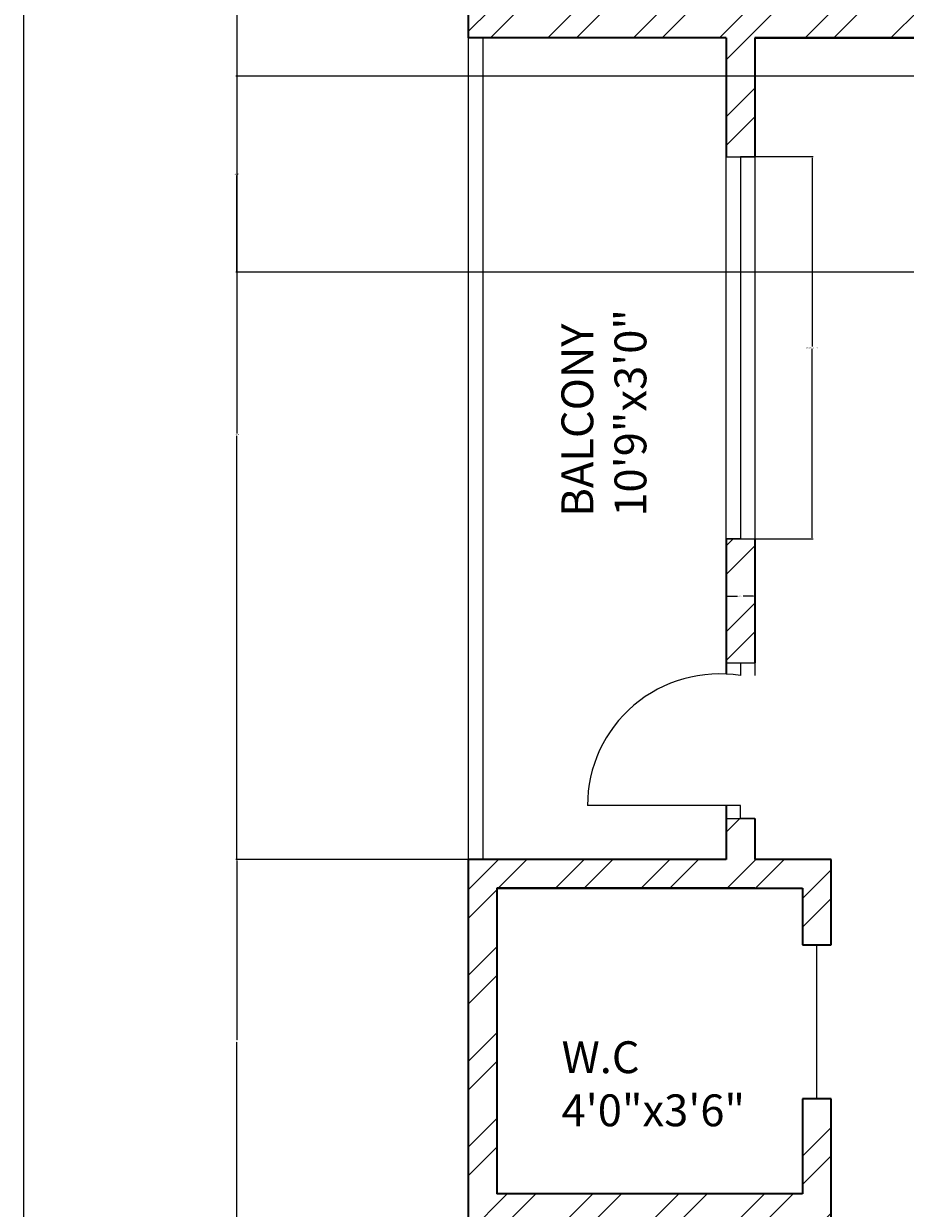
# Model space of a CAD drawing. Units: inches. Extents: x 1570 to 2186, y 1575 to 2421.
# Tile 2 of 10: x 1570 to 1708, y 1859 to 2045. Entities that reach past the tile are written whole.
import ezdxf

# ---------------------------------------------------------------- set-up
doc = ezdxf.new("R2010")
doc.units = ezdxf.units.IN
for name, color, linetype, lineweight in [('A-ANNO-DIMS', 2, 'Continuous', 18), ('A-ANNO-TTLB', 7, 'Continuous', 25), ('A-AREA-IDEN', 7, 'Continuous', 18), ('A-DOOR', 201, 'Continuous', 18), ('A-FLOR-HRAL', 201, 'Continuous', 18), ('A-GLAZ', 150, 'Continuous', 18), ('A-WALL', 7, 'Continuous', 35), ('A-WALL-PATT', 252, 'Continuous', 13)]:
    doc.layers.add(name, color=color, linetype=linetype, lineweight=lineweight)
doc.styles.get("Standard").update_dxf_attribs({"font": 'arial.ttf'})
doc.dimstyles.get("Standard").update_dxf_attribs({"dimtxt": 0.18, "dimasz": 0.18, "dimexe": 0.18, "dimexo": 0.0625, "dimgap": 0.09, "dimtad": 0, "dimtih": 1, "dimtoh": 1, "dimdec": 4, "dimzin": 0, "dimdsep": 46, "dimtxsty": 'Standard', "dimcen": 0.09, "dimadec": 0, "dimazin": 0, "dimtfac": 1, "dimtdec": 4, "dimtofl": 0, "dimtmove": 0, "dimatfit": 3, "dimfxl": 1, "dimtolj": 1, "dimtzin": 0, "dimarcsym": 0})

# ---------------------------------------------------------------- blocks, each defined once
blk = doc.blocks.new('WIN-60IN')
for p, q in [((0, 60), (4.5, 60)), ((0, 0), (0, 60)), ((4.5, 60), (2.25, 60)), ((2.25, 60), (2.25, 0)), ((4.5, 60), (4.5, 0)), ((2.25, 0), (0, 0)), ((0, 0), (4.5, 0))]:
    blk.add_line(p, q)
blk = doc.blocks.new('*D10')
at = {"layer": 'A-ANNO-DIMS', "color": 0, "lineweight": -2, "transparency": 16777216}
for p, q in [((1684.65, 2024.08), (1693.77, 2024.08)), ((1693.59, 2023.9), (1693.59, 1994.26)), ((1693.59, 1964.26), (1693.59, 1993.89)), ((1684.65, 1964.08), (1693.77, 1964.08))]:
    blk.add_line(p, q, dxfattribs=at)
at = {"layer": 'A-ANNO-DIMS', "color": 0, "transparency": 16777216}
for points in [[(1693.56, 2023.9), (1693.62, 2023.9), (1693.59, 2024.08)], [(1693.56, 1964.26), (1693.62, 1964.26), (1693.59, 1964.08)]]:
    blk.add_solid(points, dxfattribs=at)
at = {"layer": 'Defpoints', "color": 0, "transparency": 16777216}
for p in [(1684.59, 2024.08), (1693.59, 2024.08), (1684.59, 1964.08)]:
    blk.add_point(p, dxfattribs=at)
at = {"layer": 'A-ANNO-DIMS', "color": 0, "transparency": 16777216, "insert": (1693.59, 1994.08), "char_height": 0.18, "attachment_point": 5}
blk.add_mtext('\\A1;WINDOW 60 TYP.', dxfattribs=at)
blk = doc.blocks.new('*D11')
at = {"layer": 'A-ANNO-DIMS', "color": 0, "lineweight": -2, "transparency": 16777216}
for p, q in [((1680.09, 1964.01), (1680.09, 1954.9)), ((1684.59, 1964.01), (1684.59, 1954.9)), ((1680.27, 1955.08), (1681.88, 1955.08)), ((1684.41, 1955.08), (1682.8, 1955.08))]:
    blk.add_line(p, q, dxfattribs=at)
at = {"layer": 'A-ANNO-DIMS', "color": 0, "transparency": 16777216}
for points in [[(1680.27, 1955.11), (1680.27, 1955.05), (1680.09, 1955.08)], [(1684.41, 1955.11), (1684.41, 1955.05), (1684.59, 1955.08)]]:
    blk.add_solid(points, dxfattribs=at)
at = {"layer": 'Defpoints', "color": 0, "transparency": 16777216}
for p in [(1680.09, 1964.08), (1684.59, 1964.08), (1684.59, 1955.08)]:
    blk.add_point(p, dxfattribs=at)
at = {"layer": 'A-ANNO-DIMS', "color": 0, "transparency": 16777216, "insert": (1682.34, 1955.08), "char_height": 0.18, "attachment_point": 5}
blk.add_mtext('\\A1;5 TYP.', dxfattribs=at)
blk = doc.blocks.new('*D34')
at = {"layer": 'A-ANNO-DIMS', "color": 0, "lineweight": -2, "transparency": 16777216}
for p, q in [((1639.53, 1913.75), (1603.11, 1913.75)), ((1603.29, 1913.57), (1603.29, 1885.43)), ((1603.29, 1856.93), (1603.29, 1885.07)), ((1639.53, 1856.75), (1603.11, 1856.75))]:
    blk.add_line(p, q, dxfattribs=at)
at = {"layer": 'A-ANNO-DIMS', "color": 0, "transparency": 16777216}
for points in [[(1603.26, 1913.57), (1603.32, 1913.57), (1603.29, 1913.75)], [(1603.26, 1856.93), (1603.32, 1856.93), (1603.29, 1856.75)]]:
    blk.add_solid(points, dxfattribs=at)
at = {"layer": 'Defpoints', "color": 0, "transparency": 16777216}
for p in [(1603.29, 1913.75), (1639.59, 1913.75), (1639.59, 1856.75)]:
    blk.add_point(p, dxfattribs=at)
at = {"layer": 'A-ANNO-DIMS', "color": 0, "transparency": 16777216, "insert": (1603.29, 1885.25), "char_height": 0.18, "attachment_point": 5}
blk.add_mtext('\\A1;57', dxfattribs=at)
blk = doc.blocks.new('*D35')
at = {"layer": 'A-ANNO-DIMS', "color": 0, "lineweight": -2, "transparency": 16777216}
for p, q in [((1639.53, 2047.15), (1603.11, 2047.15)), ((1603.29, 2046.97), (1603.29, 1980.63)), ((1603.29, 1913.93), (1603.29, 1980.27)), ((1639.53, 1913.75), (1603.11, 1913.75))]:
    blk.add_line(p, q, dxfattribs=at)
at = {"layer": 'A-ANNO-DIMS', "color": 0, "transparency": 16777216}
for points in [[(1603.26, 2046.97), (1603.32, 2046.97), (1603.29, 2047.15)], [(1603.26, 1913.93), (1603.32, 1913.93), (1603.29, 1913.75)]]:
    blk.add_solid(points, dxfattribs=at)
at = {"layer": 'Defpoints', "color": 0, "transparency": 16777216}
for p in [(1603.29, 2047.15), (1639.59, 2047.15), (1639.59, 1913.75)]:
    blk.add_point(p, dxfattribs=at)
at = {"layer": 'A-ANNO-DIMS', "color": 0, "transparency": 16777216, "insert": (1603.29, 1980.45), "char_height": 0.18, "attachment_point": 5}
blk.add_mtext('\\A1;133.4', dxfattribs=at)
blk = doc.blocks.new('*D43')
at = {"layer": 'A-ANNO-DIMS', "color": 0, "lineweight": -2, "transparency": 16777216}
for p, q in [((1913.53, 2036.69), (1603.11, 2036.69)), ((1603.29, 2036.51), (1603.29, 2021.49)), ((1603.29, 2006.11), (1603.29, 2021.13)), ((1913.53, 2005.93), (1603.11, 2005.93))]:
    blk.add_line(p, q, dxfattribs=at)
at = {"layer": 'A-ANNO-DIMS', "color": 0, "transparency": 16777216}
for points in [[(1603.26, 2036.51), (1603.32, 2036.51), (1603.29, 2036.69)], [(1603.26, 2006.11), (1603.32, 2006.11), (1603.29, 2005.93)]]:
    blk.add_solid(points, dxfattribs=at)
at = {"layer": 'Defpoints', "color": 0, "transparency": 16777216}
for p in [(1603.29, 2036.69), (1913.59, 2036.69), (1913.59, 2005.93)]:
    blk.add_point(p, dxfattribs=at)
at = {"layer": 'A-ANNO-DIMS', "color": 0, "transparency": 16777216, "insert": (1603.29, 2021.31), "char_height": 0.18, "attachment_point": 5}
blk.add_mtext('\\A1;30.753', dxfattribs=at)

msp = doc.modelspace()

# ---------------------------------------------------------------- hatches: boundary and pattern name
at = {"layer": 'A-WALL-PATT'}
h = msp.add_hatch(dxfattribs=at)
h.set_pattern_fill('ANSI32', color=256)
h.paths.add_polyline_path([(1762.0975, 2362.1492), (1757.5975, 2362.1492), (1757.5975, 2357.6492), (1709.1163, 2357.6492), (1709.1163, 2362.1492), (1704.6163, 2362.1492), (1704.6163, 2353.1492), (1740.0886, 2353.1492), (1740.0886, 2261.8115), (1744.5886, 2261.8115), (1744.5886, 2353.1492), (1762.0975, 2353.1492)])
h.paths.add_polyline_path([(1890.2592, 2362.1492), (1885.7592, 2362.1492), (1826.5975, 2362.1492), (1822.0975, 2362.1492), (1822.0975, 2353.1492), (1862.5886, 2353.1492), (1862.5886, 2227.1492), (1744.5886, 2227.1492), (1744.5886, 2229.5389), (1742.3386, 2229.5389), (1740.0886, 2229.5389), (1740.0886, 2222.6492), (1744.5886, 2222.6492), (1756.186, 2222.6492), (1756.186, 2216.3571), (1760.686, 2216.3571), (1760.686, 2222.6492), (1832.686, 2222.6492), (1832.686, 2212.5994), (1837.186, 2212.5994), (1837.186, 2222.6492), (1893.186, 2222.6492), (1893.186, 2212.5994), (1897.686, 2212.5994), (1897.686, 2222.6492), (1989.5886, 2222.6492), (1989.5886, 2227.1492), (1989.5886, 2232.6585), (1987.3386, 2232.6585), (1985.0886, 2232.6585), (1985.0886, 2227.1492), (1867.0886, 2227.1492), (1867.0886, 2353.1492), (1890.2592, 2353.1492)])
h.paths.add_polyline_path([(1644.0886, 2353.1492), (1668.6163, 2353.1492), (1668.6163, 2362.1492), (1664.1163, 2362.1492), (1664.1163, 2358.9932), (1664.1163, 2357.6492), (1639.5886, 2357.6492), (1639.5886, 2213.8746), (1644.0886, 2213.8746), (1644.0886, 2222.6492), (1692.0886, 2222.6492), (1692.0886, 2215.9343), (1696.5886, 2215.9343), (1696.5886, 2222.6492), (1696.5886, 2227.1492), (1644.0886, 2227.1492)])
h.paths.add_polyline_path([(2013.0435, 2362.1492), (2008.5435, 2362.1492), (2008.5435, 2357.6492), (1954.7592, 2357.6492), (1954.7592, 2362.1492), (1950.2592, 2362.1492), (1950.2592, 2353.1492), (1985.0886, 2353.1492), (1985.0886, 2260.8534), (1989.5886, 2260.8534), (1989.5886, 2353.1492), (2013.0435, 2353.1492)])
h.paths.add_polyline_path([(2090.0886, 2357.6492), (2053.5435, 2357.6492), (2053.5435, 2362.1492), (2049.0435, 2362.1492), (2049.0435, 2353.1492), (2085.5886, 2353.1492), (2085.5886, 2227.1492), (2033.0886, 2227.1492), (2033.0886, 2222.6492), (2033.0886, 2214.4464), (2037.5886, 2214.4464), (2037.5886, 2222.6492), (2085.5886, 2222.6492), (2085.5886, 2212.4409), (2090.0886, 2212.4409)])
h.paths.add_polyline_path([(2090.0886, 2188.4409), (2087.8386, 2188.4409), (2085.5886, 2188.4409), (2085.5886, 2180.6492), (2037.5886, 2180.6492), (2037.5886, 2196.7956), (2033.0886, 2196.7956), (2033.0886, 2176.1492), (2037.5886, 2176.1492), (2045.0886, 2176.1492), (2045.0886, 2169.8988), (2049.5886, 2169.8988), (2049.5886, 2176.1492), (2085.5886, 2176.1492), (2085.5886, 2167.785), (2090.0886, 2167.785)])
h.paths.add_polyline_path([(2049.5886, 2147.4502), (2047.3386, 2147.4502), (2045.0886, 2147.4502), (2045.0886, 2124.4703), (2049.5886, 2124.4703)])
h.paths.add_polyline_path([(2090.0886, 2047.1492), (2049.5886, 2047.1492), (2049.5886, 2064.4703), (2045.0886, 2064.4703), (2045.0886, 2047.1492), (1918.0886, 2047.1492), (1918.0886, 2051.2061), (1913.5886, 2051.2061), (1913.5886, 2047.1492), (1913.5886, 2036.6872), (1918.0886, 2036.6872), (1918.0886, 2042.7492), (2045.0886, 2042.7492), (2045.0886, 2027.0686), (2049.5886, 2027.0686), (2049.5886, 2042.7492), (2090.0886, 2042.7492)])
h.paths.add_polyline_path([(1918.0886, 2005.9338), (1915.8386, 2005.9338), (1913.5886, 2005.9338), (1913.5886, 1913.7492), (1918.0886, 1913.7492)])
h.paths.add_polyline_path([(2090.0886, 1913.7492), (2049.5886, 1913.7492), (2045.0886, 1913.7492), (2033.0886, 1913.7492), (2033.0886, 1909.2492), (2033.0886, 1900.9803), (2037.5886, 1900.9803), (2037.5886, 1909.2492), (2085.5886, 1909.2492), (2085.5886, 1861.2492), (2037.5886, 1861.2492), (2037.5886, 1880.0859), (2033.0886, 1880.0859), (2033.0886, 1856.7492), (2085.5886, 1856.7492), (2085.5886, 1730.7492), (2054.2483, 1730.7492), (2054.2483, 1721.7492), (2058.7483, 1721.7492), (2058.7483, 1726.2492), (2090.0886, 1726.2492)])
h.paths.add_polyline_path([(2049.5886, 1967.0686), (2045.0886, 1967.0686), (2045.0886, 1913.7492), (2049.5886, 1913.7492)])
h.paths.add_polyline_path([(1989.5886, 1824.1695), (1987.3386, 1824.1695), (1985.0886, 1824.1695), (1985.0886, 1730.7492), (1989.5886, 1730.7492)])
h.paths.add_polyline_path([(1989.5886, 1861.2492), (1974.9963, 1861.2492), (1974.9963, 1865.9306), (1972.7463, 1865.9306), (1970.4963, 1865.9306), (1970.4963, 1861.2492), (1898.4963, 1861.2492), (1898.4963, 1874.2999), (1893.9963, 1874.2999), (1893.9963, 1861.2492), (1890.5886, 1861.2492), (1837.9963, 1861.2492), (1837.9963, 1874.3159), (1833.4963, 1874.3159), (1833.4963, 1861.2492), (1761.4963, 1861.2492), (1761.4963, 1865.0209), (1759.2463, 1865.0209), (1756.9963, 1865.0209), (1756.9963, 1861.2492), (1740.0886, 1861.2492), (1740.0886, 1856.7492), (1740.0886, 1850.7206), (1744.5886, 1850.7206), (1744.5886, 1856.7492), (1985.0886, 1856.7492), (1985.0886, 1851.0804), (1989.5886, 1851.0804), (1989.5886, 1856.7492)])
h.paths.add_polyline_path([(1989.5886, 1913.7492), (1740.0886, 1913.7492), (1740.0886, 1909.2492), (1756.9963, 1909.2492), (1756.9963, 1890.279), (1761.4963, 1890.279), (1761.4963, 1909.2492), (1833.4963, 1909.2492), (1833.4963, 1898.3159), (1837.9963, 1898.3159), (1837.9963, 1909.2492), (1890.5886, 1909.2492), (1893.9963, 1909.2492), (1893.9963, 1898.2999), (1898.4963, 1898.2999), (1898.4963, 1909.2492), (1970.4963, 1909.2492), (1970.4963, 1886.9887), (1974.9963, 1886.9887), (1974.9963, 1909.2492), (1989.5886, 1909.2492)])
h.paths.add_polyline_path([(1893.7344, 1730.7492), (1867.0886, 1730.7492), (1867.0886, 1856.7492), (1862.5886, 1856.7492), (1862.5886, 1730.7492), (1824.0492, 1730.7492), (1824.0492, 1721.7492), (1893.7344, 1721.7492)])
h.paths.add_polyline_path([(2018.2483, 1730.7492), (1953.7344, 1730.7492), (1953.7344, 1721.7492), (1958.2344, 1721.7492), (1958.2344, 1726.2492), (2013.7483, 1726.2492), (2013.7483, 1721.7492), (2018.2483, 1721.7492)])
h.paths.add_polyline_path([(1768.5492, 1730.7492), (1764.0492, 1730.7492), (1744.5886, 1730.7492), (1744.5886, 1819.4364), (1742.3386, 1819.4364), (1740.0886, 1819.4364), (1740.0886, 1730.7492), (1697.3801, 1730.7492), (1697.3801, 1721.7492), (1701.8801, 1721.7492), (1701.8801, 1726.2492), (1764.0492, 1726.2492), (1764.0492, 1721.7492), (1768.5492, 1721.7492)])
h.paths.add_polyline_path([(1644.0886, 1856.7492), (1639.5886, 1856.7492), (1639.5886, 1726.2492), (1657.0315, 1726.2492), (1657.0315, 1721.7492), (1661.3801, 1721.7492), (1661.3801, 1730.7492), (1644.0886, 1730.7492)])
h.paths.add_polyline_path([(1696.5886, 1876.1809), (1692.0886, 1876.1809), (1692.0886, 1861.2492), (1684.5886, 1861.2492), (1644.0886, 1861.2492), (1644.0886, 1909.2492), (1692.0886, 1909.2492), (1692.0886, 1900.3394), (1696.5886, 1900.3394), (1696.5886, 1913.7492), (1684.5886, 1913.7492), (1684.5886, 1920.2115), (1682.3386, 1920.2115), (1680.0886, 1920.2115), (1680.0886, 1913.7492), (1639.5886, 1913.7492), (1639.5886, 1856.7492), (1684.5886, 1856.7492), (1692.0886, 1856.7492), (1696.5886, 1856.7492)])
h.paths.add_polyline_path([(1684.5886, 2042.7492), (1811.5886, 2042.7492), (1811.5886, 2038.2991), (1816.0886, 2038.2991), (1816.0886, 2042.7492), (1816.0886, 2052.5708), (1813.8386, 2052.5708), (1811.5886, 2052.5708), (1811.5886, 2047.1492), (1684.5886, 2047.1492), (1684.5886, 2064.4703), (1680.0886, 2064.4703), (1680.0886, 2047.1492), (1639.5886, 2047.1492), (1639.5886, 2042.7492), (1680.0886, 2042.7492), (1680.0886, 2024.0762), (1684.5886, 2024.0762)])
h.paths.add_polyline_path([(1684.5886, 1964.0762), (1680.0886, 1964.0762), (1680.0886, 1944.6145), (1684.5886, 1944.6145)])
h.paths.add_polyline_path([(1816.0886, 1973.7492), (1876.0886, 1973.7492), (1876.0886, 1959.17), (1880.5886, 1959.17), (1880.5886, 1973.7492), (1880.5886, 1978.2492), (1816.0886, 1978.2492), (1816.0886, 2005.9338), (1813.8386, 2005.9338), (1811.5886, 2005.9338), (1811.5886, 1913.7492), (1816.0886, 1913.7492)])
h.paths.add_polyline_path([(1837.186, 2180.6492), (1837.186, 2188.5994), (1834.936, 2188.5994), (1832.686, 2188.5994), (1832.686, 2180.6492), (1760.686, 2180.6492), (1760.686, 2197.4807), (1756.186, 2197.4807), (1756.186, 2180.6492), (1744.5886, 2180.6492), (1740.0886, 2180.6492), (1740.0886, 2176.1492), (1837.186, 2176.1492)])
h.paths.add_polyline_path([(1974.186, 2196.8744), (1971.936, 2196.8744), (1969.686, 2196.8744), (1969.686, 2180.6492), (1897.686, 2180.6492), (1897.686, 2188.5994), (1895.436, 2188.5994), (1893.186, 2188.5994), (1893.186, 2180.6492), (1893.186, 2176.1492), (1974.186, 2176.1492)])
h.paths.add_polyline_path([(1918.0886, 2176.1492), (1913.5886, 2176.1492), (1913.5886, 2081.3709), (1918.0886, 2081.3709)])
h.paths.add_polyline_path([(1816.0886, 2176.1492), (1811.5886, 2176.1492), (1811.5886, 2081.3709), (1816.0886, 2081.3709)])
h.paths.add_polyline_path([(1684.5886, 2150.4939), (1682.3386, 2150.4939), (1680.0886, 2150.4939), (1680.0886, 2124.4703), (1684.5886, 2124.4703)])
h.paths.add_polyline_path([(1696.5886, 2180.6492), (1696.5886, 2197.4701), (1692.0886, 2197.4701), (1692.0886, 2180.6492), (1644.0886, 2180.6492), (1644.0886, 2189.8746), (1641.8386, 2189.8746), (1639.5886, 2189.8746), (1639.5886, 2169.814), (1644.0886, 2169.814), (1644.0886, 2176.1492), (1680.0886, 2176.1492), (1680.0886, 2171.7002), (1684.5886, 2171.7002), (1684.5886, 2176.1492), (1696.5886, 2176.1492)])

# ---------------------------------------------------------------- linework, layer by layer
at = {"layer": 'A-ANNO-TTLB'}
msp.add_lwpolyline([(1569.8198, 2421.0436), (2186.3437, 2421.0436), (2186.3437, 1574.5084), (1569.8198, 1574.5084)], close=True, dxfattribs=at)
at = {"layer": 'A-DOOR'}
for p, q in [((1680.0886, 1944.6145), (1684.5886, 1944.6145)), ((1682.3386, 1944.6145), (1682.3386, 1942.6145)), ((1684.5886, 1944.6145), (1684.5886, 1942.6145)), ((1682.3386, 1922.2115), (1658.3386, 1922.2115)), ((1682.3386, 1920.2115), (1682.3386, 1922.2115)), ((1680.0886, 1920.2115), (1684.5886, 1920.2115)), ((1684.5886, 1920.2115), (1682.3386, 1920.2115)), ((1694.3386, 1876.1809), (1694.3386, 1900.3394))]:
    msp.add_line(p, q, dxfattribs=at)
msp.add_arc((1679.0112, 1922.2115), 20.6726, 80.737505, 180, dxfattribs=at)
at = {"layer": 'A-FLOR-HRAL'}
for p, q in [((1639.5886, 2042.7492), (1639.5886, 1913.7492)), ((1641.9287, 2042.7492), (1641.9287, 1913.7492))]:
    msp.add_line(p, q, dxfattribs=at)
at = {"layer": 'A-WALL'}
for p, q in [((1639.5886, 2047.1492), (1639.5886, 2042.7492)), ((1680.0886, 2042.7492), (1639.5886, 2042.7492)), ((1680.0886, 2042.7492), (1680.0886, 2024.0762)), ((1684.5886, 2042.7492), (1684.5886, 2024.0762)), ((1684.5886, 2042.7492), (1811.5886, 2042.7492)), ((1811.5886, 2042.7492), (1684.5886, 2042.7492)), ((1680.0886, 1964.0762), (1680.0886, 1942.856)), ((1684.5886, 1964.0762), (1684.5886, 1944.6145)), ((1680.0886, 1922.2115), (1680.0886, 1913.7492)), ((1684.5886, 1920.2115), (1684.5886, 1913.7492)), ((1680.0886, 1913.7492), (1639.5886, 1913.7492)), ((1639.5886, 1913.7492), (1639.5886, 1726.2492)), ((1680.0886, 1913.7492), (1644.0886, 1913.7492)), ((1696.5886, 1913.7492), (1684.5886, 1913.7492)), ((1696.5886, 1900.3394), (1696.5886, 1913.7492)), ((1684.5886, 1909.2492), (1644.0886, 1909.2492)), ((1644.0886, 1909.2492), (1692.0886, 1909.2492)), ((1644.0886, 1909.2492), (1644.0886, 1861.2492)), ((1692.0886, 1909.2492), (1692.0886, 1900.3394)), ((1692.0886, 1900.3394), (1696.5886, 1900.3394)), ((1696.5886, 1876.1809), (1692.0886, 1876.1809)), ((1692.0886, 1876.1809), (1692.0886, 1861.2492)), ((1696.5886, 1856.7492), (1696.5886, 1876.1809)), ((1684.5886, 1861.2492), (1644.0886, 1861.2492)), ((1692.0886, 1861.2492), (1684.5886, 1861.2492))]:
    msp.add_line(p, q, dxfattribs=at)

# ---------------------------------------------------------------- block references
at = {"layer": 'A-GLAZ'}
msp.add_blockref('WIN-60IN', (1680.089, 1964.076), dxfattribs=at)

# ---------------------------------------------------------------- texts
at = {"layer": 'A-AREA-IDEN', "insert": (1654.2489, 1967.5718), "char_height": 5, "attachment_point": 1, "rotation": 90}
msp.add_mtext_dynamic_manual_height_columns('BALCONY\\P10\'9"x3\'0"', width=152.484585, gutter_width=12.5, heights=[0], dxfattribs=at)
at = {"layer": 'A-AREA-IDEN', "insert": (1654.2758, 1885.2146), "char_height": 5, "attachment_point": 1}
msp.add_mtext_dynamic_manual_height_columns('W.C\\P4\'0"x3\'6"', width=106.332724, gutter_width=12.5, heights=[0], dxfattribs=at)

# ---------------------------------------------------------------- dimensions: what is measured, and where the dimension line sits
at = {"layer": 'A-ANNO-DIMS'}
for base, p1, p2, override, picture, middle in [((1603.2886, 2047.1492), (1639.5886, 1913.7492), (1639.5886, 2047.1492), {"dimdec": 1, "dimlfac": 1, "dimrnd": 0, "dimzin": 0, "dimdsep": 46, "dimlunit": 2}, '*D35', (1603.2886, 1980.4492)), ((1603.2886, 2036.6872), (1913.5886, 2005.9338), (1913.5886, 2036.6872), {"dimdec": 3, "dimlfac": 1, "dimrnd": 0, "dimzin": 0, "dimdsep": 46, "dimlunit": 2}, '*D43', (1603.2886, 2021.3105)), ((1603.2886, 1913.7492), (1639.5886, 1856.7492), (1639.5886, 1913.7492), {"dimdec": 0, "dimlfac": 1, "dimrnd": 0, "dimzin": 0, "dimdsep": 46, "dimlunit": 2}, '*D34', (1603.2886, 1885.2492))]:
    dim = msp.add_linear_dim(base=base, p1=p1, p2=p2, angle=90, dimstyle='Standard', override=override, dxfattribs=at)
    dim.commit()
    dim.dimension.update_dxf_attribs({"geometry": picture, "text_midpoint": middle})
dim = msp.add_linear_dim(base=(1693.5886, 2024.0762), p1=(1684.5886, 1964.0762), p2=(1684.5886, 2024.0762), angle=90, text='WINDOW <> TYP.', dimstyle='Standard', override={"dimdec": 0, "dimlfac": 1, "dimrnd": 0, "dimzin": 0, "dimdsep": 46, "dimlunit": 2}, dxfattribs=at)
dim.commit()
dim.dimension.update_dxf_attribs({"geometry": '*D10', "text_midpoint": (1693.5886, 1994.0762)})
dim = msp.add_linear_dim(base=(1684.5886393898, 1955.0761936205), p1=(1680.0886393898, 1964.0761936205), p2=(1684.5886393898, 1964.0761936205), text='<> TYP.', dimstyle='Standard', override={"dimdec": 0, "dimlfac": 1, "dimrnd": 0, "dimzin": 0, "dimdsep": 46, "dimlunit": 2}, dxfattribs=at)
dim.commit()
dim.dimension.update_dxf_attribs({"geometry": '*D11', "text_midpoint": (1682.3386393898, 1955.0761936205)})

doc.saveas('drawing.dxf')
